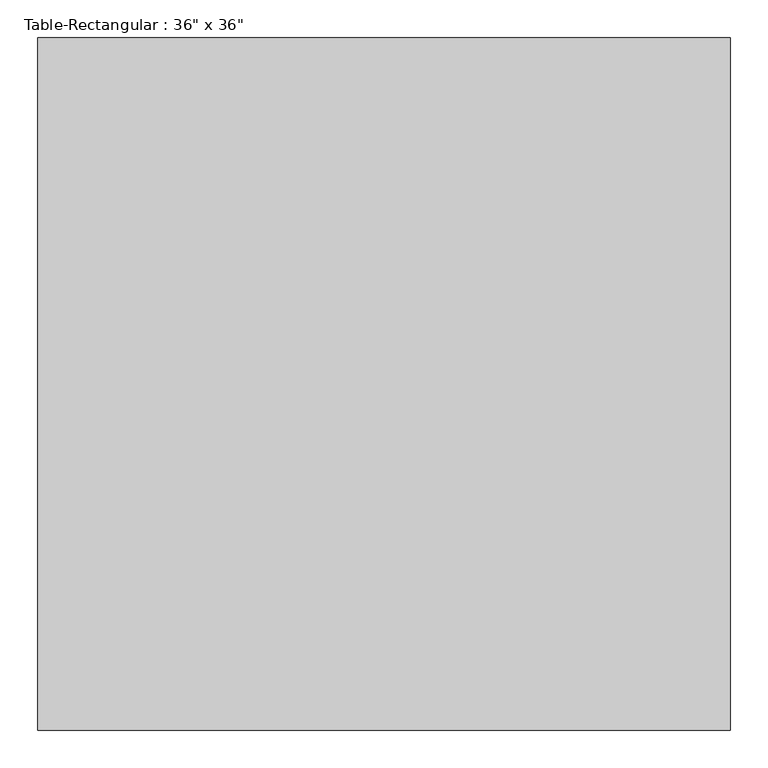
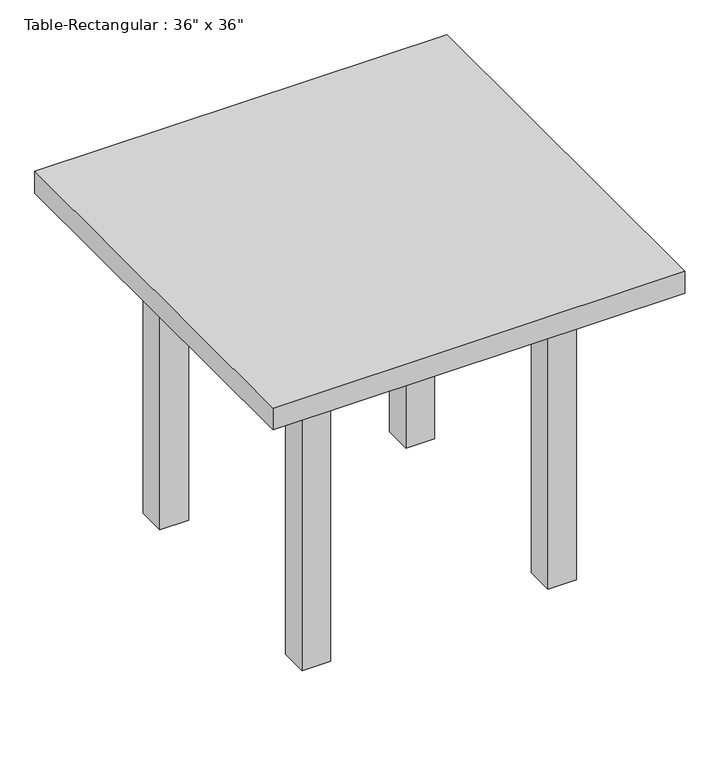
"""IFC4 building model written with IfcOpenShell, lengths in millimetres: furniture geometry."""

from ifc_helpers import new_model, si_unit, frame, origin, origin_with_axes, place, context, project, spatial, polyline, outline, extrude, source, transform, mapped, element, save


def furniture_4d44e21c(model_context):
    return source(origin(), model_context, "Body", "SweptSolid", [
        extrude(outline(polyline([(241.3, 266.7), (241.3, 241.3), (-241.3, 241.3), (-241.3, 266.7), (241.3, 266.7)])), frame((0.0, 0.0, 609.6), z_axis=(0.0, 0.0, 1.0), x_axis=(1.0, 0.0, 0.0)), (0.0, 0.0, 1.0), 101.6),
        extrude(outline(polyline([(241.3, -266.7), (-241.3, -266.7), (-241.3, -241.3), (241.3, -241.3), (241.3, -266.7)])), frame((0.0, 0.0, 609.6), z_axis=(0.0, 0.0, 1.0), x_axis=(1.0, 0.0, 0.0)), (0.0, 0.0, 1.0), 101.6),
        extrude(outline(polyline([(-254.0, -241.3), (-279.4, -241.3), (-279.4, 241.3), (-254.0, 241.3), (-254.0, -241.3)])), frame((0.0, 0.0, 609.6), z_axis=(0.0, 0.0, 1.0), x_axis=(1.0, 0.0, 0.0)), (0.0, 0.0, 1.0), 101.6),
        extrude(outline(polyline([(254.0, -241.3), (254.0, 241.3), (279.4, 241.3), (279.4, -241.3), (254.0, -241.3)])), frame((0.0, 0.0, 609.6), z_axis=(0.0, 0.0, 1.0), x_axis=(1.0, 0.0, 0.0)), (0.0, 0.0, 1.0), 101.6),
        extrude(outline(polyline([(457.2, 457.2), (457.2, -457.2), (-457.2, -457.2), (-457.2, 457.2), (457.2, 457.2)])), frame((0.0, 0.0, 711.2), z_axis=(0.0, 0.0, 1.0), x_axis=(1.0, 0.0, 0.0)), (0.0, 0.0, 1.0), 50.8),
        extrude(outline(polyline([(-241.3, 304.8), (-241.3, 241.3), (-304.8, 241.3), (-304.8, 304.8), (-241.3, 304.8)])), origin_with_axes(), (0.0, 0.0, 1.0), 711.2),
        extrude(outline(polyline([(241.3, 304.8), (304.8, 304.8), (304.8, 241.3), (241.3, 241.3), (241.3, 304.8)])), origin_with_axes(), (0.0, 0.0, 1.0), 711.2),
        extrude(outline(polyline([(-241.3, -304.8), (-304.8, -304.8), (-304.8, -241.3), (-241.3, -241.3), (-241.3, -304.8)])), origin_with_axes(), (0.0, 0.0, 1.0), 711.2),
        extrude(outline(polyline([(241.3, -304.8), (241.3, -241.3), (304.8, -241.3), (304.8, -304.8), (241.3, -304.8)])), origin_with_axes(), (0.0, 0.0, 1.0), 711.2),
    ])


if __name__ == "__main__":
    model = new_model("IFC4")
    model_context = context("Model", 3, world=origin())
    ifc_project = project(units=[si_unit("LENGTHUNIT", "METRE", prefix="MILLI")], contexts=[model_context])
    site = spatial("IfcSite", under=ifc_project)
    building = spatial("IfcBuilding", under=site)
    placement = place(None, origin())
    furniture_shape = furniture_4d44e21c(model_context)
    element("IfcFurniture", 1, ObjectType="Table-Rectangular : 36\" x 36\"", at=placement, inside=building, context=model_context, shape_type="MappedRepresentation", body=[
        mapped(furniture_shape, transform((0.0, 0.0, 0.0), x_axis=(1.0, 0.0, 0.0), y_axis=(0.0, 1.0, 0.0), z_axis=(0.0, 0.0, 1.0))),
    ])
    save(model, "model.ifc")

# Revit data of these elements
# Type "Table-Rectangular : 36\" x 36\""
#   Assembly Code = "E2020200"
#   Height = 2' - 6"
#   Length = 3' - 0"
#   Width = 3' - 0"
#   Base Material = Birch
#   Top Material = Birch
# Element 1 (IfcFurniture, "Table-Rectangular : 36\" x 36\"")
#   Materials on its faces: "Birch"
# Materials
#   "Birch": class "Wood", colour RGB 224 178 126, transparency 0, Description = "Betula Alleghaniensis", Cost = 0
